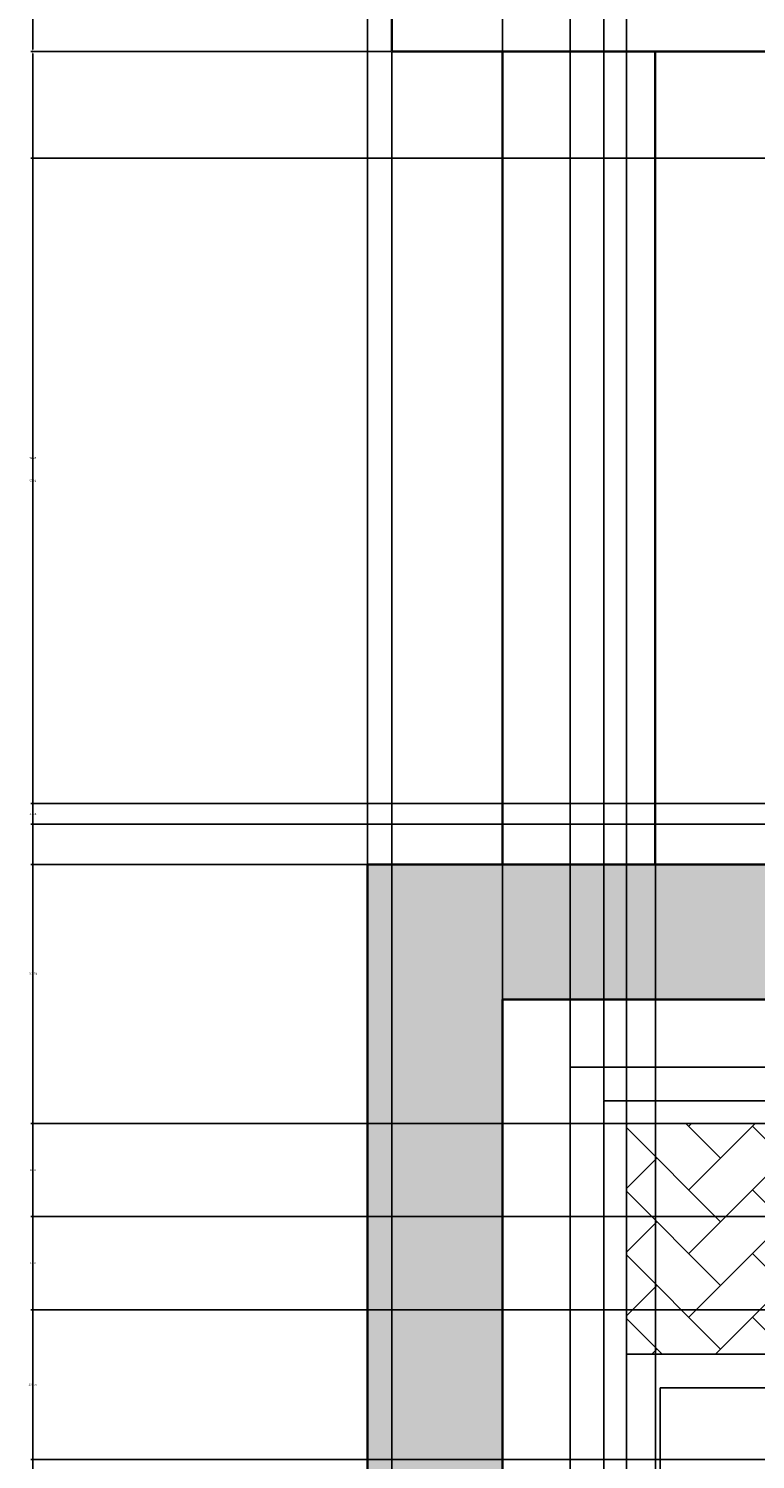
# Model space of a CAD drawing. Units: inches. Extents: x -13 to 630, y -103 to 275.
# Tile 3 of 9: x -13 to 51, y 72 to 199. Entities that reach past the tile are written whole.
import ezdxf

# ---------------------------------------------------------------- set-up
doc = ezdxf.new("R2010")
doc.units = ezdxf.units.IN
doc.header["$MEASUREMENT"] = 0
for name, color, linetype, lineweight in [('A-ANNO-DIMS', 2, 'Continuous', 18), ('A-ELEV', 7, 'Continuous', 35), ('A-ELEV-PATT', 8, 'Continuous', 13), ('A-GLAZ', 4, 'Continuous', 25)]:
    doc.layers.add(name, color=color, linetype=linetype, lineweight=lineweight)
doc.styles.get("Standard").update_dxf_attribs({"font": 'arial.ttf'})
doc.dimstyles.get("Standard").update_dxf_attribs({"dimtxt": 0.18, "dimasz": 0.18, "dimexe": 0.18, "dimexo": 0.0625, "dimgap": 0.09, "dimtad": 0, "dimtih": 1, "dimtoh": 1, "dimdec": 4, "dimzin": 0, "dimdsep": 46, "dimtxsty": 'Standard', "dimcen": 0.09, "dimadec": 0, "dimazin": 0, "dimtfac": 1, "dimtdec": 4, "dimtofl": 0, "dimtmove": 0, "dimatfit": 3, "dimfxl": 1, "dimtolj": 1, "dimtzin": 0, "dimarcsym": 0})

# ---------------------------------------------------------------- blocks, each defined once
blk = doc.blocks.new('WIN-GROUND')
for points in [[(0, 0), (0, 102), (108, 102), (108, 0)], [(3, 0), (3, 99), (105, 99), (105, 0)], [(5, 0), (5, 97), (103, 97), (103, 0)], [(34.74, 56.82), (34.74, 73.49), (37, 73.49), (37, 56.82)], [(73.43, 56.82), (73.43, 73.49), (75.7, 73.49), (75.7, 56.82)], [(34.74, 55.51), (8, 55.51), (8, 56.82), (34.74, 56.82)], [(37, 56.82), (73.43, 56.82)], [(75.7, 56.82), (100, 56.82), (100, 55.51), (75.7, 55.51)], [(34.74, 21.58), (34.74, 55.51)], [(37, 55.51), (37, 21.58)], [(73.43, 55.51), (37, 55.51)], [(73.43, 21.58), (73.43, 55.51)], [(75.7, 55.51), (75.7, 21.58)], [(34.74, 20.27), (8, 20.27), (8, 21.58), (34.74, 21.58)], [(37, 21.58), (73.43, 21.58)], [(75.7, 21.58), (100, 21.58), (100, 20.27), (75.7, 20.27)], [(37, 20.27), (37, 3), (34.74, 3), (34.74, 20.27)], [(73.43, 20.27), (37, 20.27)], [(75.7, 20.27), (75.7, 3), (73.43, 3), (73.43, 20.27)]]:
    blk.add_lwpolyline(points)
for points in [[(5, 97), (103, 97), (103, 76.49), (5, 76.49)], [(5, 76.49), (103, 76.49), (103, 0), (5, 0)], [(8, 73.49), (100, 73.49), (100, 3), (8, 3)]]:
    blk.add_lwpolyline(points, close=True)
blk = doc.blocks.new('*D7')
at = {"layer": 'A-ANNO-DIMS', "color": 0, "lineweight": -2, "transparency": 16777216}
for p, q in [((16.71, 5.14), (16.71, 275.01)), ((16.89, 274.83), (25.5, 274.83)), ((34.53, 274.83), (25.92, 274.83)), ((34.71, 5.14), (34.71, 275.01))]:
    blk.add_line(p, q, dxfattribs=at)
at = {"layer": 'A-ANNO-DIMS', "color": 0, "transparency": 16777216}
for points in [[(16.89, 274.86), (16.89, 274.8), (16.71, 274.83)], [(34.53, 274.86), (34.53, 274.8), (34.71, 274.83)]]:
    blk.add_solid(points, dxfattribs=at)
at = {"layer": 'Defpoints', "color": 0, "transparency": 16777216}
for p in [(34.71, 274.83), (16.71, 5.08), (34.71, 5.08)]:
    blk.add_point(p, dxfattribs=at)
at = {"layer": 'A-ANNO-DIMS', "color": 0, "transparency": 16777216, "insert": (25.71, 274.83), "char_height": 0.18, "attachment_point": 5}
blk.add_mtext('\\A1;18', dxfattribs=at)
blk = doc.blocks.new('*D12')
at = {"layer": 'A-ANNO-DIMS', "color": 0, "lineweight": -2, "transparency": 16777216}
for p, q in [((16.65, 125.08), (-13.22, 125.08)), ((-13.04, 124.9), (-13.04, 65.26)), ((-13.04, 5.26), (-13.04, 64.9)), ((16.65, 5.08), (-13.22, 5.08))]:
    blk.add_line(p, q, dxfattribs=at)
at = {"layer": 'A-ANNO-DIMS', "color": 0, "transparency": 16777216}
for points in [[(-13.07, 124.9), (-13.01, 124.9), (-13.04, 125.08)], [(-13.07, 5.26), (-13.01, 5.26), (-13.04, 5.08)]]:
    blk.add_solid(points, dxfattribs=at)
at = {"layer": 'Defpoints', "color": 0, "transparency": 16777216}
for p in [(-13.04, 125.08), (16.71, 125.08), (16.71, 5.08)]:
    blk.add_point(p, dxfattribs=at)
at = {"layer": 'A-ANNO-DIMS', "color": 0, "transparency": 16777216, "insert": (-13.04, 65.08), "char_height": 0.18, "attachment_point": 5}
blk.add_mtext('\\A1;120', dxfattribs=at)
blk = doc.blocks.new('*D41')
at = {"layer": 'A-ANNO-DIMS', "color": 0, "lineweight": -2, "transparency": 16777216}
for p, q in [((205.96, 72.22), (-13.22, 72.22)), ((-13.04, 72.04), (-13.04, 71.07)), ((-13.04, 69.73), (-13.04, 70.7)), ((205.96, 69.55), (-13.22, 69.55))]:
    blk.add_line(p, q, dxfattribs=at)
at = {"layer": 'A-ANNO-DIMS', "color": 0, "transparency": 16777216}
for points in [[(-13.07, 72.04), (-13.01, 72.04), (-13.04, 72.22)], [(-13.07, 69.73), (-13.01, 69.73), (-13.04, 69.55)]]:
    blk.add_solid(points, dxfattribs=at)
at = {"layer": 'Defpoints', "color": 0, "transparency": 16777216}
for p in [(-13.04, 72.22), (206.02, 72.22), (206.02, 69.55)]:
    blk.add_point(p, dxfattribs=at)
at = {"layer": 'A-ANNO-DIMS', "color": 0, "transparency": 16777216, "insert": (-13.04, 70.88), "char_height": 0.18, "attachment_point": 5}
blk.add_mtext('\\A1;2.68', dxfattribs=at)
blk = doc.blocks.new('*D42')
at = {"layer": 'A-ANNO-DIMS', "color": 0, "lineweight": -2, "transparency": 16777216}
for p, q in [((205.96, 85.52), (-13.22, 85.52)), ((-13.04, 85.34), (-13.04, 79.05)), ((-13.04, 72.4), (-13.04, 78.69)), ((205.96, 72.22), (-13.22, 72.22))]:
    blk.add_line(p, q, dxfattribs=at)
at = {"layer": 'A-ANNO-DIMS', "color": 0, "transparency": 16777216}
for points in [[(-13.07, 85.34), (-13.01, 85.34), (-13.04, 85.52)], [(-13.07, 72.4), (-13.01, 72.4), (-13.04, 72.22)]]:
    blk.add_solid(points, dxfattribs=at)
at = {"layer": 'Defpoints', "color": 0, "transparency": 16777216}
for p in [(-13.04, 85.52), (206.02, 85.52), (206.02, 72.22)]:
    blk.add_point(p, dxfattribs=at)
at = {"layer": 'A-ANNO-DIMS', "color": 0, "transparency": 16777216, "insert": (-13.04, 78.87), "char_height": 0.18, "attachment_point": 5}
blk.add_mtext('\\A1;13.297', dxfattribs=at)
blk = doc.blocks.new('*D43')
at = {"layer": 'A-ANNO-DIMS', "color": 0, "lineweight": -2, "transparency": 16777216}
for p, q in [((205.96, 93.8), (-13.22, 93.8)), ((-13.04, 93.62), (-13.04, 89.84)), ((-13.04, 85.7), (-13.04, 89.48)), ((205.96, 85.52), (-13.22, 85.52))]:
    blk.add_line(p, q, dxfattribs=at)
at = {"layer": 'A-ANNO-DIMS', "color": 0, "transparency": 16777216}
for points in [[(-13.07, 93.62), (-13.01, 93.62), (-13.04, 93.8)], [(-13.07, 85.7), (-13.01, 85.7), (-13.04, 85.52)]]:
    blk.add_solid(points, dxfattribs=at)
at = {"layer": 'Defpoints', "color": 0, "transparency": 16777216}
for p in [(-13.04, 93.8), (206.02, 93.8), (206.02, 85.52)]:
    blk.add_point(p, dxfattribs=at)
at = {"layer": 'A-ANNO-DIMS', "color": 0, "transparency": 16777216, "insert": (-13.04, 89.66), "char_height": 0.18, "attachment_point": 5}
blk.add_mtext('\\A1;8.28', dxfattribs=at)
blk = doc.blocks.new('*D44')
at = {"layer": 'A-ANNO-DIMS', "color": 0, "lineweight": -2, "transparency": 16777216}
for p, q in [((205.96, 102.08), (-13.22, 102.08)), ((-13.04, 101.9), (-13.04, 98.12)), ((-13.04, 93.98), (-13.04, 97.76)), ((205.96, 93.8), (-13.22, 93.8))]:
    blk.add_line(p, q, dxfattribs=at)
at = {"layer": 'A-ANNO-DIMS', "color": 0, "transparency": 16777216}
for points in [[(-13.07, 101.9), (-13.01, 101.9), (-13.04, 102.08)], [(-13.07, 93.98), (-13.01, 93.98), (-13.04, 93.8)]]:
    blk.add_solid(points, dxfattribs=at)
at = {"layer": 'Defpoints', "color": 0, "transparency": 16777216}
for p in [(-13.04, 102.08), (206.02, 102.08), (206.02, 93.8)]:
    blk.add_point(p, dxfattribs=at)
at = {"layer": 'A-ANNO-DIMS', "color": 0, "transparency": 16777216, "insert": (-13.04, 97.94), "char_height": 0.18, "attachment_point": 5}
blk.add_mtext('\\A1;8.28', dxfattribs=at)
blk = doc.blocks.new('*D45')
at = {"layer": 'A-ANNO-DIMS', "color": 0, "lineweight": -2, "transparency": 16777216}
for p, q in [((205.96, 128.66), (-13.22, 128.66)), ((-13.04, 128.48), (-13.04, 115.55)), ((-13.04, 102.26), (-13.04, 115.19)), ((205.96, 102.08), (-13.22, 102.08))]:
    blk.add_line(p, q, dxfattribs=at)
at = {"layer": 'A-ANNO-DIMS', "color": 0, "transparency": 16777216}
for points in [[(-13.07, 128.48), (-13.01, 128.48), (-13.04, 128.66)], [(-13.07, 102.26), (-13.01, 102.26), (-13.04, 102.08)]]:
    blk.add_solid(points, dxfattribs=at)
at = {"layer": 'Defpoints', "color": 0, "transparency": 16777216}
for p in [(-13.04, 128.66), (206.02, 128.66), (206.02, 102.08)]:
    blk.add_point(p, dxfattribs=at)
at = {"layer": 'A-ANNO-DIMS', "color": 0, "transparency": 16777216, "insert": (-13.04, 115.37), "char_height": 0.18, "attachment_point": 5}
blk.add_mtext('\\A1;26.574', dxfattribs=at)
blk = doc.blocks.new('*D46')
at = {"layer": 'A-ANNO-DIMS', "color": 0, "lineweight": -2, "transparency": 16777216}
for p, q in [((205.96, 130.51), (-13.22, 130.51)), ((-13.04, 130.33), (-13.04, 129.76)), ((205.96, 128.66), (-13.22, 128.66)), ((-13.04, 128.84), (-13.04, 129.4))]:
    blk.add_line(p, q, dxfattribs=at)
at = {"layer": 'A-ANNO-DIMS', "color": 0, "transparency": 16777216}
for points in [[(-13.07, 130.33), (-13.01, 130.33), (-13.04, 130.51)], [(-13.07, 128.84), (-13.01, 128.84), (-13.04, 128.66)]]:
    blk.add_solid(points, dxfattribs=at)
at = {"layer": 'Defpoints', "color": 0, "transparency": 16777216}
for p in [(-13.04, 130.51), (206.02, 130.51), (206.02, 128.66)]:
    blk.add_point(p, dxfattribs=at)
at = {"layer": 'A-ANNO-DIMS', "color": 0, "transparency": 16777216, "insert": (-13.04, 129.58), "char_height": 0.18, "attachment_point": 5}
blk.add_mtext('\\A1;1.854', dxfattribs=at)
blk = doc.blocks.new('*D47')
at = {"layer": 'A-ANNO-DIMS', "color": 0, "lineweight": -2, "transparency": 16777216}
for p, q in [((252.21, 187.83), (-13.22, 187.83)), ((-13.04, 187.65), (-13.04, 159.35)), ((-13.04, 130.69), (-13.04, 158.99)), ((205.96, 130.51), (-13.22, 130.51))]:
    blk.add_line(p, q, dxfattribs=at)
at = {"layer": 'A-ANNO-DIMS', "color": 0, "transparency": 16777216}
for points in [[(-13.07, 187.65), (-13.01, 187.65), (-13.04, 187.83)], [(-13.07, 130.69), (-13.01, 130.69), (-13.04, 130.51)]]:
    blk.add_solid(points, dxfattribs=at)
at = {"layer": 'Defpoints', "color": 0, "transparency": 16777216}
for p in [(-13.04, 187.83), (252.27, 187.83), (206.02, 130.51)]:
    blk.add_point(p, dxfattribs=at)
at = {"layer": 'A-ANNO-DIMS', "color": 0, "transparency": 16777216, "insert": (-13.04, 159.17), "char_height": 0.18, "attachment_point": 5}
blk.add_mtext('\\A1;57.32', dxfattribs=at)
blk = doc.blocks.new('*D67')
at = {"layer": 'A-ANNO-DIMS', "color": 0, "lineweight": -2, "transparency": 16777216}
for p, q in [((28.71, 113.14), (28.71, 275.01)), ((28.89, 274.83), (31.56, 274.83)), ((34.53, 274.83), (31.86, 274.83)), ((34.71, 107.14), (34.71, 275.01))]:
    blk.add_line(p, q, dxfattribs=at)
at = {"layer": 'A-ANNO-DIMS', "color": 0, "transparency": 16777216}
for points in [[(28.89, 274.86), (28.89, 274.8), (28.71, 274.83)], [(34.53, 274.86), (34.53, 274.8), (34.71, 274.83)]]:
    blk.add_solid(points, dxfattribs=at)
at = {"layer": 'Defpoints', "color": 0, "transparency": 16777216}
for p in [(34.71, 274.83), (28.71, 113.08), (34.71, 107.08)]:
    blk.add_point(p, dxfattribs=at)
at = {"layer": 'A-ANNO-DIMS', "color": 0, "transparency": 16777216, "insert": (31.71, 274.83), "char_height": 0.18, "attachment_point": 5}
blk.add_mtext('\\A1;6', dxfattribs=at)
blk = doc.blocks.new('*D68')
at = {"layer": 'A-ANNO-DIMS', "color": 0, "lineweight": -2, "transparency": 16777216}
for p, q in [((34.71, 107.14), (34.71, 275.01)), ((34.89, 274.83), (36.06, 274.83)), ((37.53, 274.83), (36.36, 274.83)), ((37.71, 104.14), (37.71, 275.01))]:
    blk.add_line(p, q, dxfattribs=at)
at = {"layer": 'A-ANNO-DIMS', "color": 0, "transparency": 16777216}
for points in [[(34.89, 274.86), (34.89, 274.8), (34.71, 274.83)], [(37.53, 274.86), (37.53, 274.8), (37.71, 274.83)]]:
    blk.add_solid(points, dxfattribs=at)
at = {"layer": 'Defpoints', "color": 0, "transparency": 16777216}
for p in [(37.71, 274.83), (34.71, 107.08), (37.71, 104.08)]:
    blk.add_point(p, dxfattribs=at)
at = {"layer": 'A-ANNO-DIMS', "color": 0, "transparency": 16777216, "insert": (36.21, 274.83), "char_height": 0.18, "attachment_point": 5}
blk.add_mtext('\\A1;3', dxfattribs=at)
blk = doc.blocks.new('*D69')
at = {"layer": 'A-ANNO-DIMS', "color": 0, "lineweight": -2, "transparency": 16777216}
for p, q in [((37.71, 104.14), (37.71, 275.01)), ((37.89, 274.83), (38.56, 274.83)), ((39.53, 274.83), (38.86, 274.83)), ((39.71, 102.14), (39.71, 275.01))]:
    blk.add_line(p, q, dxfattribs=at)
at = {"layer": 'A-ANNO-DIMS', "color": 0, "transparency": 16777216}
for points in [[(37.89, 274.86), (37.89, 274.8), (37.71, 274.83)], [(39.53, 274.86), (39.53, 274.8), (39.71, 274.83)]]:
    blk.add_solid(points, dxfattribs=at)
at = {"layer": 'Defpoints', "color": 0, "transparency": 16777216}
for p in [(39.71, 274.83), (37.71, 104.08), (39.71, 102.08)]:
    blk.add_point(p, dxfattribs=at)
at = {"layer": 'A-ANNO-DIMS', "color": 0, "transparency": 16777216, "insert": (38.71, 274.83), "char_height": 0.18, "attachment_point": 5}
blk.add_mtext('\\A1;2', dxfattribs=at)
blk = doc.blocks.new('*D87')
at = {"layer": 'A-ANNO-DIMS', "color": 0, "lineweight": -2, "transparency": 16777216}
for p, q in [((18.81, 197.32), (-13.22, 197.32)), ((-13.04, 197.14), (-13.04, 161.38)), ((-13.04, 125.26), (-13.04, 161.02)), ((16.65, 125.08), (-13.22, 125.08))]:
    blk.add_line(p, q, dxfattribs=at)
at = {"layer": 'A-ANNO-DIMS', "color": 0, "transparency": 16777216}
for points in [[(-13.07, 197.14), (-13.01, 197.14), (-13.04, 197.32)], [(-13.07, 125.26), (-13.01, 125.26), (-13.04, 125.08)]]:
    blk.add_solid(points, dxfattribs=at)
at = {"layer": 'Defpoints', "color": 0, "transparency": 16777216}
for p in [(-13.04, 197.32), (18.87, 197.32), (16.71, 125.08)]:
    blk.add_point(p, dxfattribs=at)
at = {"layer": 'A-ANNO-DIMS', "color": 0, "transparency": 16777216, "insert": (-13.04, 161.2), "char_height": 0.18, "attachment_point": 5}
blk.add_mtext('\\A1;72.24', dxfattribs=at)
blk = doc.blocks.new('*D88')
at = {"layer": 'A-ANNO-DIMS', "color": 0, "lineweight": -2, "transparency": 16777216}
for p, q in [((18.81, 206.53), (-13.22, 206.53)), ((-13.04, 206.35), (-13.04, 202.11)), ((-13.04, 197.5), (-13.04, 201.74)), ((18.81, 197.32), (-13.22, 197.32))]:
    blk.add_line(p, q, dxfattribs=at)
at = {"layer": 'A-ANNO-DIMS', "color": 0, "transparency": 16777216}
for points in [[(-13.07, 206.35), (-13.01, 206.35), (-13.04, 206.53)], [(-13.07, 197.5), (-13.01, 197.5), (-13.04, 197.32)]]:
    blk.add_solid(points, dxfattribs=at)
at = {"layer": 'Defpoints', "color": 0, "transparency": 16777216}
for p in [(-13.04, 206.53), (18.87, 206.53), (18.87, 197.32)]:
    blk.add_point(p, dxfattribs=at)
at = {"layer": 'A-ANNO-DIMS', "color": 0, "transparency": 16777216, "insert": (-13.04, 201.92), "char_height": 0.18, "attachment_point": 5}
blk.add_mtext('\\A1;9.206', dxfattribs=at)
blk = doc.blocks.new('*D95')
at = {"layer": 'A-ANNO-DIMS', "color": 0, "lineweight": -2, "transparency": 16777216}
for p, q in [((16.71, 125.14), (16.71, 275.01)), ((16.89, 274.83), (17.47, 274.83)), ((18.69, 274.83), (18.12, 274.83)), ((18.87, 206.59), (18.87, 275.01))]:
    blk.add_line(p, q, dxfattribs=at)
at = {"layer": 'A-ANNO-DIMS', "color": 0, "transparency": 16777216}
for points in [[(16.89, 274.86), (16.89, 274.8), (16.71, 274.83)], [(18.69, 274.86), (18.69, 274.8), (18.87, 274.83)]]:
    blk.add_solid(points, dxfattribs=at)
at = {"layer": 'Defpoints', "color": 0, "transparency": 16777216}
for p in [(18.87, 274.83), (18.87, 206.53), (16.71, 125.08)]:
    blk.add_point(p, dxfattribs=at)
at = {"layer": 'A-ANNO-DIMS', "color": 0, "transparency": 16777216, "insert": (17.79, 274.83), "char_height": 0.18, "attachment_point": 5}
blk.add_mtext('\\A1;2.16', dxfattribs=at)
blk = doc.blocks.new('*D103')
at = {"layer": 'A-ANNO-DIMS', "color": 0, "lineweight": -2, "transparency": 16777216}
for p, q in [((18.87, 197.26), (18.87, -103.45)), ((28.71, 197.26), (28.71, -103.45)), ((19.05, -103.27), (23.4, -103.27)), ((28.53, -103.27), (24.19, -103.27))]:
    blk.add_line(p, q, dxfattribs=at)
at = {"layer": 'A-ANNO-DIMS', "color": 0, "transparency": 16777216}
for points in [[(19.05, -103.24), (19.05, -103.3), (18.87, -103.27)], [(28.53, -103.24), (28.53, -103.3), (28.71, -103.27)]]:
    blk.add_solid(points, dxfattribs=at)
at = {"layer": 'Defpoints', "color": 0, "transparency": 16777216}
for p in [(18.87, 197.32), (28.71, 197.32), (28.71, -103.27)]:
    blk.add_point(p, dxfattribs=at)
at = {"layer": 'A-ANNO-DIMS', "color": 0, "transparency": 16777216, "insert": (23.79, -103.27), "char_height": 0.18, "attachment_point": 5}
blk.add_mtext('\\A1;9.838', dxfattribs=at)
blk = doc.blocks.new('*D104')
at = {"layer": 'A-ANNO-DIMS', "color": 0, "lineweight": -2, "transparency": 16777216}
for p, q in [((16.71, 125.02), (16.71, -103.45)), ((28.71, 125.02), (28.71, -103.45)), ((16.89, -103.27), (22.5, -103.27)), ((28.53, -103.27), (22.92, -103.27))]:
    blk.add_line(p, q, dxfattribs=at)
at = {"layer": 'A-ANNO-DIMS', "color": 0, "transparency": 16777216}
for points in [[(16.89, -103.24), (16.89, -103.3), (16.71, -103.27)], [(28.53, -103.24), (28.53, -103.3), (28.71, -103.27)]]:
    blk.add_solid(points, dxfattribs=at)
at = {"layer": 'Defpoints', "color": 0, "transparency": 16777216}
for p in [(16.71, 125.08), (28.71, 125.08), (28.71, -103.27)]:
    blk.add_point(p, dxfattribs=at)
at = {"layer": 'A-ANNO-DIMS', "color": 0, "transparency": 16777216, "insert": (22.71, -103.27), "char_height": 0.18, "attachment_point": 5}
blk.add_mtext('\\A1;12', dxfattribs=at)
blk = doc.blocks.new('*D105')
at = {"layer": 'A-ANNO-DIMS', "color": 0, "lineweight": -2, "transparency": 16777216}
for p, q in [((28.71, 125.02), (28.71, -103.45)), ((42.29, 125.02), (42.29, -103.45)), ((28.89, -103.27), (35.04, -103.27)), ((42.11, -103.27), (35.95, -103.27))]:
    blk.add_line(p, q, dxfattribs=at)
at = {"layer": 'A-ANNO-DIMS', "color": 0, "transparency": 16777216}
for points in [[(28.89, -103.24), (28.89, -103.3), (28.71, -103.27)], [(42.11, -103.24), (42.11, -103.3), (42.29, -103.27)]]:
    blk.add_solid(points, dxfattribs=at)
at = {"layer": 'Defpoints', "color": 0, "transparency": 16777216}
for p in [(28.71, 125.08), (42.29, 125.08), (42.29, -103.27)]:
    blk.add_point(p, dxfattribs=at)
at = {"layer": 'A-ANNO-DIMS', "color": 0, "transparency": 16777216, "insert": (35.5, -103.27), "char_height": 0.18, "attachment_point": 5}
blk.add_mtext('\\A1;13.574', dxfattribs=at)
blk = doc.blocks.new('*D106')
at = {"layer": 'A-ANNO-DIMS', "color": 0, "lineweight": -2, "transparency": 16777216}
for p, q in [((42.29, 125.02), (42.29, -103.45)), ((53, 125.02), (53, -103.45)), ((42.47, -103.27), (47.27, -103.27)), ((52.82, -103.27), (48.01, -103.27))]:
    blk.add_line(p, q, dxfattribs=at)
at = {"layer": 'A-ANNO-DIMS', "color": 0, "transparency": 16777216}
for points in [[(42.47, -103.24), (42.47, -103.3), (42.29, -103.27)], [(52.82, -103.24), (52.82, -103.3), (53, -103.27)]]:
    blk.add_solid(points, dxfattribs=at)
at = {"layer": 'Defpoints', "color": 0, "transparency": 16777216}
for p in [(42.29, 125.08), (53, 125.08), (53, -103.27)]:
    blk.add_point(p, dxfattribs=at)
at = {"layer": 'A-ANNO-DIMS', "color": 0, "transparency": 16777216, "insert": (47.64, -103.27), "char_height": 0.18, "attachment_point": 5}
blk.add_mtext('\\A1;10.71', dxfattribs=at)

msp = doc.modelspace()

# ---------------------------------------------------------------- hatches: boundary and pattern name
at = {"layer": 'A-ELEV-PATT'}
h = msp.add_hatch(dxfattribs=at)
h.set_pattern_fill('BRSTONE', color=256, scale=20)
h.paths.add_polyline_path([(120.6641, 172.7854), (64.9953, 172.7854, 0.41421356), (54.9953, 162.7854), (54.9953, 125.0808), (59.9953, 125.0808), (59.9953, 162.7854, -0.41421356), (64.9953, 167.7854), (120.6641, 167.7854, -0.41421356), (125.6641, 162.7854), (125.6641, 125.0808), (130.6641, 125.0808), (130.6641, 162.7854, 0.41421356)])
h.paths.add_polyline_path([(439.5513, 172.7854), (383.8825, 172.7854, 0.41421356), (373.8825, 162.7854), (373.8825, 125.0808), (378.8825, 125.0808), (378.8825, 162.7854, -0.41421356), (383.8825, 167.7854), (439.5513, 167.7854, -0.41421356), (444.5513, 162.7854), (444.5513, 125.0808), (449.5513, 125.0808), (449.5513, 162.7854, 0.41421356)])
h.paths.add_polyline_path([(364.7117, 113.0808), (484.7117, 113.0808), (484.7117, 5.0808), (496.7117, 5.0808), (496.7117, 125.0808), (345.3061, 125.0808), (345.3061, 5.0808), (364.7117, 5.0808)])
h.paths.add_polyline_path([(164.8443, 125.0808), (28.7117, 125.0808), (16.7117, 125.0808), (16.7117, 5.0808), (28.7117, 5.0808), (28.7117, 113.0808), (148.7117, 113.0808), (148.7117, 5.0808), (164.8443, 5.0808)])
h.paths.add_polyline_path([(95.1171, 223.9392), (83.8622, 223.9392), (83.8622, 206.5279), (95.1171, 206.5279)])
h.paths.add_polyline_path([(54.9212, 223.9392), (40.7186, 223.9392), (40.7186, 206.5279), (54.9212, 206.5279)])
h.paths.add_polyline_path([(463.828, 223.9392), (449.6254, 223.9392), (449.6254, 206.5279), (463.828, 206.5279)])
h.paths.add_polyline_path([(420.6843, 223.9392), (409.4295, 223.9392), (409.4295, 206.5279), (420.6843, 206.5279)])
h = msp.add_hatch(dxfattribs=at)
h.set_pattern_fill('AR-HBONE', color=256)
h.paths.add_polyline_path([(137.7117, 102.0808), (39.7117, 102.0808), (39.7117, 81.5713), (137.7117, 81.5713)])
h.paths.add_polyline_path([(473.7117, 102.0808), (375.7117, 102.0808), (375.7117, 81.5713), (473.7117, 81.5713)])

# ---------------------------------------------------------------- linework, layer by layer
at = {"layer": 'A-ELEV'}
msp.add_line((42.2856, 125.0808), (42.2856, 197.3216), dxfattribs=at)
for points in [[(18.8732, 197.3216), (164.8443, 197.3216), (164.8443, 206.5279), (18.8732, 206.5279)], [(28.7117, 125.0808), (164.8443, 125.0808), (164.8443, 197.3216), (28.7117, 197.3216)]]:
    msp.add_lwpolyline(points, close=True, dxfattribs=at)
for points in [[(164.8443, 125.0808), (16.7117, 125.0808), (16.7117, 5.0808)], [(28.7117, 5.0808), (28.7117, 113.0808), (148.7117, 113.0808), (148.7117, 5.0808)]]:
    msp.add_lwpolyline(points, dxfattribs=at)

# ---------------------------------------------------------------- block references
at = {"layer": 'A-GLAZ'}
msp.add_blockref('WIN-GROUND', (34.712, 5.081), dxfattribs=at)

# ---------------------------------------------------------------- dimensions: what is measured, and where the dimension line sits
at = {"layer": 'A-ANNO-DIMS'}
for base, p1, p2, override, picture, middle in [((34.7117, 274.8308), (16.7117, 5.0808), (34.7117, 5.0808), {"dimdec": 0, "dimlfac": 1, "dimrnd": 0, "dimzin": 0, "dimdsep": 46, "dimlunit": 2}, '*D7', (25.7117, 274.8308)), ((18.8732, 274.8308), (16.7117, 125.0808), (18.8732, 206.5279), {"dimdec": 2, "dimlfac": 1, "dimrnd": 0, "dimzin": 0, "dimdsep": 46, "dimlunit": 2}, '*D95', (17.7925, 274.8308)), ((34.7117, 274.8308), (28.7117, 113.0808), (34.7117, 107.0808), {"dimdec": 0, "dimlfac": 1, "dimrnd": 0, "dimzin": 0, "dimdsep": 46, "dimlunit": 2}, '*D67', (31.7117, 274.8308)), ((37.7117, 274.8308), (34.7117, 107.0808), (37.7117, 104.0808), {"dimdec": 0, "dimlfac": 1, "dimrnd": 0, "dimzin": 0, "dimdsep": 46, "dimlunit": 2}, '*D68', (36.2117, 274.8308)), ((39.7117, 274.8308), (37.7117, 104.0808), (39.7117, 102.0808), {"dimdec": 0, "dimlfac": 1, "dimrnd": 0, "dimzin": 0, "dimdsep": 46, "dimlunit": 2}, '*D69', (38.7117, 274.8308)), ((28.71172, -103.27457), (18.87325, 197.32155), (28.71172, 197.32155), {"dimdec": 3, "dimlfac": 1, "dimrnd": 0, "dimzin": 0, "dimdsep": 46, "dimlunit": 2}, '*D103', (23.79248, -103.27457)), ((28.7117, -103.2746), (16.7117, 125.0808), (28.7117, 125.0808), {"dimdec": 0, "dimlfac": 1, "dimrnd": 0, "dimzin": 0, "dimdsep": 46, "dimlunit": 2}, '*D104', (22.7117, -103.2746)), ((42.2856, -103.2746), (28.7117, 125.0808), (42.2856, 125.0808), {"dimdec": 3, "dimlfac": 1, "dimrnd": 0, "dimzin": 0, "dimdsep": 46, "dimlunit": 2}, '*D105', (35.4987, -103.2746)), ((52.9953, -103.2746), (42.2856, 125.0808), (52.9953, 125.0808), {"dimdec": 2, "dimlfac": 1, "dimrnd": 0, "dimzin": 0, "dimdsep": 46, "dimlunit": 2}, '*D106', (47.6404, -103.2746))]:
    dim = msp.add_linear_dim(base=base, p1=p1, p2=p2, dimstyle='Standard', override=override, dxfattribs=at)
    dim.commit()
    dim.dimension.update_dxf_attribs({"geometry": picture, "text_midpoint": middle})
for base, p1, p2, override, picture, middle in [((-13.0383, 206.5279), (18.8732, 197.3216), (18.8732, 206.5279), {"dimdec": 3, "dimlfac": 1, "dimrnd": 0, "dimzin": 0, "dimdsep": 46, "dimlunit": 2}, '*D88', (-13.0383, 201.9247)), ((-13.0383, 197.3216), (16.7117, 125.0808), (18.8732, 197.3216), {"dimdec": 2, "dimlfac": 1, "dimrnd": 0, "dimzin": 0, "dimdsep": 46, "dimlunit": 2}, '*D87', (-13.0383, 161.2012)), ((-13.0383, 187.8302), (206.0208, 130.5093), (252.2733, 187.8302), {"dimdec": 2, "dimlfac": 1, "dimrnd": 0, "dimzin": 0, "dimdsep": 46, "dimlunit": 2}, '*D47', (-13.0383, 159.1697)), ((-13.0383, 130.5093), (206.0208, 128.6551), (206.0208, 130.5093), {"dimdec": 3, "dimlfac": 1, "dimrnd": 0, "dimzin": 0, "dimdsep": 46, "dimlunit": 2}, '*D46', (-13.0383, 129.5822)), ((-13.0383, 128.6551), (206.0208, 102.0808), (206.0208, 128.6551), {"dimdec": 3, "dimlfac": 1, "dimrnd": 0, "dimzin": 0, "dimdsep": 46, "dimlunit": 2}, '*D45', (-13.0383, 115.368)), ((-13.0383, 125.0808), (16.7117, 5.0808), (16.7117, 125.0808), {"dimdec": 0, "dimlfac": 1, "dimrnd": 0, "dimzin": 0, "dimdsep": 46, "dimlunit": 2}, '*D12', (-13.0383, 65.0808)), ((-13.0383, 102.0808), (206.0208, 93.8005), (206.0208, 102.0808), {"dimdec": 2, "dimlfac": 1, "dimrnd": 0, "dimzin": 0, "dimdsep": 46, "dimlunit": 2}, '*D44', (-13.0383, 97.9406)), ((-13.0383, 93.8005), (206.0208, 85.5202), (206.0208, 93.8005), {"dimdec": 2, "dimlfac": 1, "dimrnd": 0, "dimzin": 0, "dimdsep": 46, "dimlunit": 2}, '*D43', (-13.0383, 89.6603)), ((-13.0383, 85.5202), (206.0208, 72.223), (206.0208, 85.5202), {"dimdec": 3, "dimlfac": 1, "dimrnd": 0, "dimzin": 0, "dimdsep": 46, "dimlunit": 2}, '*D42', (-13.0383, 78.8716)), ((-13.0383, 72.223), (206.0208, 69.5455), (206.0208, 72.223), {"dimdec": 2, "dimlfac": 1, "dimrnd": 0, "dimzin": 0, "dimdsep": 46, "dimlunit": 2}, '*D41', (-13.0383, 70.8842))]:
    dim = msp.add_linear_dim(base=base, p1=p1, p2=p2, angle=90, dimstyle='Standard', override=override, dxfattribs=at)
    dim.commit()
    dim.dimension.update_dxf_attribs({"geometry": picture, "text_midpoint": middle})

doc.saveas('drawing.dxf')
